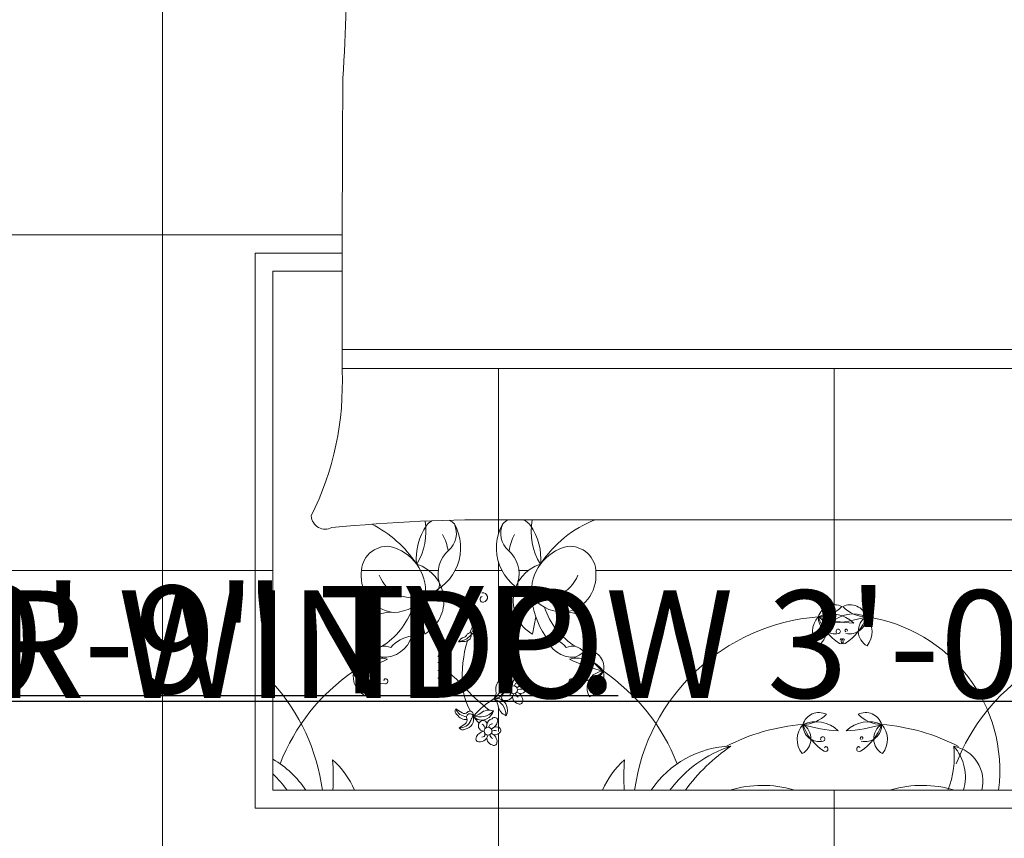
# Model space of a CAD drawing. Units: inches. Extents: x 351 to 1738, y -265 to 286.
# Tile 23 of 38: x 1127 to 1200, y 41 to 102. Entities that reach past the tile are written whole.
import ezdxf

# ---------------------------------------------------------------- set-up
doc = ezdxf.new("R2010")
doc.units = ezdxf.units.IN
doc.header["$MEASUREMENT"] = 0
for name, color, linetype, lineweight in [('A-ANNO-DIMS', 2, 'Continuous', 18), ('A-FLOR-PATT', 9, 'Continuous', 9), ('A-FURN', 18, 'Continuous', 13)]:
    doc.layers.add(name, color=color, linetype=linetype, lineweight=lineweight)
doc.styles.get("Standard").update_dxf_attribs({"font": 'arial.ttf'})
doc.dimstyles.get("Standard").update_dxf_attribs({"dimtxt": 8, "dimasz": 5, "dimexe": 0.18, "dimexo": 0.0625, "dimgap": 0.09, "dimtad": 1, "dimtoh": 1, "dimzin": 0, "dimdsep": 46, "dimlunit": 4, "dimtxsty": 'Standard', "dimcen": 0, "dimclre": 256, "dimadec": 0, "dimazin": 0, "dimtfac": 1, "dimtofl": 0, "dimtmove": 0, "dimatfit": 3, "dimfxl": 1, "dimtolj": 1, "dimtzin": 0, "dimlwe": -1, "dimarcsym": 0})

# ---------------------------------------------------------------- blocks, each defined once
blk = doc.blocks.new('*D52')
at = {"layer": 'A-ANNO-DIMS', "color": 0, "lineweight": -2, "transparency": 16777216}
for p, q in [((1098.304, 46.258), (1098.304, 51.258)), ((1098.304, 51.258), (1235.278, 51.258)), ((1098.304, 15.258), (1098.304, 41.258))]:
    blk.add_line(p, q, dxfattribs=at)
at = {"layer": 'A-ANNO-DIMS', "transparency": 16777216}
for p, q in [((1103.642, 46.258), (1098.124, 46.258)), ((1103.642, 10.258), (1098.124, 10.258))]:
    blk.add_line(p, q, dxfattribs=at)
at = {"layer": 'A-ANNO-DIMS', "color": 0, "transparency": 16777216}
for points in [[(1097.471, 41.258), (1099.137, 41.258), (1098.304, 46.258)], [(1097.471, 15.258), (1099.137, 15.258), (1098.304, 10.258)]]:
    blk.add_solid(points, dxfattribs=at)
at = {"layer": 'Defpoints', "color": 0, "transparency": 16777216}
for p in [(1098.304, 46.258), (1103.704, 46.258), (1103.704, 10.258)]:
    blk.add_point(p, dxfattribs=at)
at = {"layer": 'A-ANNO-DIMS', "color": 0, "transparency": 16777216, "insert": (1166.836, 55.49), "char_height": 8, "attachment_point": 5}
blk.add_mtext('\\A1;STAIR WINDOW 3\'-0" TYP.', dxfattribs=at)
blk = doc.blocks.new('*D53')
at = {"layer": 'A-ANNO-DIMS', "color": 0, "lineweight": -2, "transparency": 16777216}
for p, q in [((1098.704, 51.658), (1093.704, 51.658)), ((1117.704, 51.658), (1171.648, 51.658))]:
    blk.add_line(p, q, dxfattribs=at)
at = {"layer": 'A-ANNO-DIMS', "transparency": 16777216}
for p, q in [((1103.704, 46.321), (1103.704, 51.838)), ((1112.704, 46.321), (1112.704, 51.838))]:
    blk.add_line(p, q, dxfattribs=at)
at = {"layer": 'A-ANNO-DIMS', "color": 0, "transparency": 16777216}
for points in [[(1098.704, 52.492), (1098.704, 50.825), (1103.704, 51.658)], [(1117.704, 52.492), (1117.704, 50.825), (1112.704, 51.658)]]:
    blk.add_solid(points, dxfattribs=at)
at = {"layer": 'Defpoints', "color": 0, "transparency": 16777216}
for p in [(1112.704, 51.658), (1103.704, 46.258), (1112.704, 46.258)]:
    blk.add_point(p, dxfattribs=at)
at = {"layer": 'A-ANNO-DIMS', "color": 0, "transparency": 16777216, "insert": (1147.176, 55.833), "char_height": 8, "attachment_point": 5}
blk.add_mtext('\\A1;0\'-9" TYP.', dxfattribs=at)

msp = doc.modelspace()

# ---------------------------------------------------------------- hatches: boundary and pattern name
at = {"layer": 'A-FLOR-PATT', "transparency": 33554559}
h = msp.add_hatch(dxfattribs=at)
h.set_pattern_fill('ANSI37', color=256, scale=200, angle=135)
h.set_pattern_definition([(180, (1112.704, -164.037), (-2e-15, -25), []), (270, (1112.704, -164.037), (25, -5e-15), [])])
h.paths.add_polyline_path([(1380.064, 73.463), (1380.132, 148.463), (1338.064, 148.463), (1290.704, 148.463), (1290.704, 88.463), (1248.704, 88.463), (1248.704, -2.009), (1244.704, -2.009), (1244.704, 142.457), (1160.704, 142.457), (1160.704, 158.963), (1160.704, 170.137), (1160.704, 206.137), (1160.704, 228.963), (1112.704, 228.963), (1112.704, 209.963), (1112.704, 168.963), (1124.704, 168.963), (1124.704, 162.963), (1112.704, 162.963), (1112.704, 64.463), (1112.704, 60.463), (1112.704, 0.463), (1112.704, -48.026), (1146.804, -47.981), (1146.804, -35.691), (1207.804, -35.691), (1207.804, -47.902), (1236.542, -47.864), (1236.544, -50.009), (1248.5, -50.009), (1248.506, -102.915), (1248.512, -150.915), (1248.514, -164.037), (1248.549, -164.037), (1273.017, -164.037), (1273.017, -128.799), (1355.24, -128.799), (1355.24, -164.037), (1384.204, -164.037), (1384.204, -57.037), (1380.064, -57.037), (1380.064, -48.037), (1392.064, -48.037), (1392.064, -53.037), (1406.549, -53.037), (1406.549, -57.037), (1401.204, -57.037), (1401.204, -147.037), (1468.204, -147.037), (1468.204, -138.5), (1472.204, -138.5), (1472.204, -102.5), (1468.204, -102.5), (1468.204, -57.037), (1442.549, -57.037), (1442.549, -53.037), (1463.049, -53.037), (1463.049, -40.747), (1524.049, -40.747), (1524.049, -48.037), (1536.064, -48.037), (1536.064, -53.037), (1557.704, -53.037), (1557.704, 204.963), (1384.204, 204.963), (1384.204, 73.463), (1392.064, 73.463), (1392.064, 64.463), (1384.204, 64.463), (1384.204, -3.5), (1380.204, -3.537), (1380.204, 64.463), (1380.064, 64.463)])
h.paths.add_polyline_path([(1510.714, 86.458, -0.103984), (1511.661, 85.595, 0.470438), (1510.158, 87.614, 0.0961)], flags=16)
h.paths.add_polyline_path([(1510.443, 100.266, 0.009798), (1504.693, 100.48, 0.02879), (1504.6, 99.767, -0.165331), (1505.519, 96.135, -0.143601)], flags=16)
h.paths.add_polyline_path([(1487.201, 85.595, -0.103984), (1488.148, 86.458, 0.0961), (1488.704, 87.614, 0.470438)], flags=0)
h.paths.add_polyline_path([(1495.052, 100.43), (1494.178, 100.43, -0.026463), (1494.262, 99.774, -0.144219)], flags=16)
h.paths.add_polyline_path([(1444.485, 86.458, -0.103984), (1445.433, 85.595, 0.470438), (1443.93, 87.614, 0.0961)], flags=16)
h.paths.add_polyline_path([(1420.972, 85.595, -0.103984), (1421.92, 86.458, 0.0961), (1422.475, 87.614, 0.470438)], flags=16)
h.paths.add_polyline_path([(1428.632, 100.335, 0.001054), (1427.971, 100.309, -0.021524), (1428.033, 99.774, -0.114301)], flags=16)
h.paths.add_polyline_path([(1419.906, 143.708, 0.024979), (1420.222, 157.526), (1421.573, 159.101), (1421.573, 175.369), (1391.393, 175.369), (1391.393, 200.519), (1542.294, 200.519), (1542.294, 175.369), (1512.028, 175.369, 0.019865), (1511.521, 153.838, 0.025134), (1512.758, 118.323, 0.020553), (1512.942, 115.253), (1419.834, 115.253, -0.000414), (1419.843, 124.798), (1413.059, 124.798), (1413.059, 84.437, -0.061853), (1415.831, 80.45, -0.093077), (1420.972, 85.595, -0.267537), (1422.371, 84.732, 0.08511), (1424.052, 84.616, -0.885393), (1424.033, 84.851, -1.125815), (1424.073, 84.366, -0.087987), (1422.371, 84.732, -0.267537), (1422.326, 83.089, -0.370542), (1420.972, 85.595, 0.093077), (1415.831, 80.45, -0.087414), (1417.914, 73.937), (1418.941, 73.937, 0.02725), (1418.913, 76.906, -0.115703), (1421.051, 73.937), (1445.354, 73.937, -0.115703), (1447.492, 76.906, 0.02725), (1447.464, 73.937), (1448.491, 73.937, -0.087414), (1450.574, 80.45, 0.093077), (1445.433, 85.595, -0.370542), (1444.079, 83.089, -0.267537), (1444.034, 84.732, -0.087987), (1442.332, 84.366, -1.125815), (1442.372, 84.851, -2.032736), (1442.364, 84.368, 0.086378), (1444.034, 84.732, -0.267537), (1445.433, 85.595, -0.093077), (1450.574, 80.45, -0.257732), (1466.483, 90.927, -0.47867), (1468.832, 91.907, -0.47867), (1471.18, 90.927, -0.26264), (1483.053, 81.78, -0.071866), (1487.201, 85.595, -0.267537), (1488.6, 84.732, 0.08511), (1490.28, 84.616, -0.885393), (1490.262, 84.851, -1.125815), (1490.301, 84.366, -0.087987), (1488.6, 84.732, -0.267537), (1488.554, 83.089, -0.370542), (1487.201, 85.595, 0.071866), (1483.053, 81.78, -0.132065), (1484.143, 73.937), (1485.169, 73.937, 0.02725), (1485.142, 76.906, -0.115703), (1487.28, 73.937), (1511.582, 73.937, -0.115703), (1513.72, 76.906, 0.02725), (1513.693, 73.937), (1514.719, 73.937, -0.087414), (1516.802, 80.45, 0.093077), (1511.661, 85.595, -0.370542), (1510.308, 83.089, -0.267537), (1510.262, 84.732, -0.087987), (1508.561, 84.366, -1.125815), (1508.601, 84.851, -2.032736), (1508.592, 84.368, 0.086378), (1510.262, 84.732, -0.267537), (1511.661, 85.595, -0.093077), (1516.802, 80.45, -0.061853), (1519.575, 84.437), (1519.575, 73.937), (1413.059, 73.937), (1413.059, 124.798), (1419.843, 124.798, -0.000821)], flags=16)
h.paths.add_polyline_path([(1220.149, 54.133, -0.103984), (1220.869, 53.476, 0.470438), (1219.727, 55.011, 0.0961)], flags=16)
h.paths.add_polyline_path([(1219.944, 64.626, 0.009798), (1215.574, 64.789, 0.02879), (1215.503, 64.247, -0.165331), (1216.201, 61.487, -0.143601)], flags=16)
h.paths.add_polyline_path([(1209.779, 64.449, 0.097446), (1209.339, 64.751), (1208.247, 64.751, 0.12739), (1207.7, 64.326, 0.171586), (1206.95, 61.475, -0.158854), (1207.636, 59.45, 0.015898), (1207.795, 59.218, 0.061546), (1208.598, 59.616, 0.175416), (1208.638, 60.099, -0.284779), (1209.348, 62.472, 0.326216)], flags=16)
h.paths.add_polyline_path([(1169.818, 54.133, -0.103984), (1170.538, 53.476, 0.470438), (1169.396, 55.011, 0.0961)], flags=16)
h.paths.add_polyline_path([(1159.017, 62.472, 0.284764), (1158.307, 60.099, -0.175433), (1158.267, 59.616, 0.39293), (1159.448, 64.449, -0.32623)], flags=16)
h.paths.add_polyline_path([(1156.342, 58.239, -0.178321), (1154.011, 55.31, -0.174736), (1154.722, 55.233, -0.200802), (1156.27, 56.086, 0.12699), (1157.283, 58.991, -0.091205)], flags=16)
h.paths.add_polyline_path([(1156.624, 61.413, 0.157275), (1157.316, 64.247, 0.169622)], flags=16)
h.paths.add_polyline_path([(1152.67, 54.133, -0.0961), (1151.95, 53.476, 0.064076), (1154.465, 54.384, 0.199016)], flags=16)
h.paths.add_polyline_path([(1202.281, 53.476, -0.103984), (1203, 54.133, 0.0961), (1203.423, 55.011, 0.470438)], flags=0)
h.paths.add_polyline_path([(1151.139, 97.64, 0.024979), (1151.379, 108.141), (1152.406, 109.338), (1152.406, 121.701), (1129.47, 121.701), (1129.47, 140.814), (1244.149, 140.814), (1244.149, 121.701), (1221.148, 121.701, 0.019865), (1220.763, 105.338, 0.025134), (1221.703, 78.349, 0.020553), (1221.843, 76.016), (1151.078, 76.016, -0.128743), (1148.786, 65.037, 0.539352), (1150.327, 64.171, -0.027594), (1163.481, 64.751, 0.097695), (1163.04, 64.449, 0.326216), (1163.471, 62.472, -0.284777), (1164.181, 60.099, -0.194757), (1165.846, 61.443, -0.155402), (1165.172, 64.247, -0.166022), (1165.869, 61.475, -0.177014), (1167.852, 62.77, -0.448203), (1169.974, 60.807, -0.393499), (1167.679, 57.86, -0.895548), (1168.438, 54.524, -0.355767), (1166.218, 56.086, -0.066024), (1165.505, 57.539), (1165.251, 56.243, -0.371732), (1164.02, 59.758, -0.373614), (1163.04, 64.449, -0.097695), (1163.481, 64.751, 0.021354), (1153.294, 64.429, -0.134183), (1156.695, 61.368, 0.186873), (1154.636, 62.77, 0.448203), (1152.514, 60.807, 0.403726), (1154.905, 57.846, 0.711219), (1153.334, 55, 0.53154), (1151.95, 53.476, -0.267537), (1153.013, 52.821, 0.08511), (1154.29, 52.732, -0.885393), (1154.276, 52.911, -1.125815), (1154.306, 52.543, -0.087987), (1153.013, 52.821, -0.267537), (1152.978, 51.572, -0.370542), (1151.95, 53.476, 0.093077), (1148.043, 49.566, -0.087414), (1149.626, 44.617), (1150.406, 44.617, 0.02725), (1150.385, 46.873, -0.115703), (1152.01, 44.617), (1170.478, 44.617, -0.115703), (1172.103, 46.873, 0.02725), (1172.082, 44.617), (1172.862, 44.617, -0.087414), (1174.445, 49.566, 0.093077), (1170.538, 53.476, -0.370542), (1169.51, 51.572, -0.267537), (1169.475, 52.821, -0.087987), (1168.182, 52.543, -1.125815), (1168.212, 52.911, -2.032736), (1168.206, 52.544, 0.086378), (1169.475, 52.821, -0.267537), (1170.538, 53.476, -0.093077), (1174.445, 49.566, -0.257732), (1186.536, 57.528, -0.47867), (1188.321, 58.273, -0.47867), (1190.106, 57.528, -0.26264), (1199.128, 50.577, -0.071866), (1202.281, 53.476, -0.267537), (1203.344, 52.821, 0.08511), (1204.621, 52.732, -0.885393), (1204.607, 52.911, -1.125815), (1204.637, 52.543, -0.087987), (1203.344, 52.821, -0.267537), (1203.309, 51.572, -0.370542), (1202.281, 53.476, 0.071866), (1199.128, 50.577, -0.132065), (1199.957, 44.617), (1200.737, 44.617, 0.02725), (1200.716, 46.873, -0.115703), (1202.341, 44.617), (1220.809, 44.617, -0.115703), (1222.434, 46.873, 0.02725), (1222.413, 44.617), (1223.193, 44.617, -0.087414), (1224.776, 49.566, 0.093077), (1220.869, 53.476, -0.370542), (1219.841, 51.572, -0.267537), (1219.806, 52.821, -0.087987), (1218.513, 52.543, -1.125815), (1218.543, 52.911, -2.032736), (1218.537, 52.544, 0.086378), (1219.806, 52.821, -0.267537), (1220.869, 53.476, -0.093077), (1224.776, 49.566, -0.061853), (1226.883, 52.597), (1226.883, 44.617), (1145.936, 44.617), (1145.936, 83.269), (1151.091, 83.269, -0.000821)], flags=16)
h.paths.add_polyline_path([(1218.01, 57.86, -0.895548), (1218.769, 54.524, -0.355767), (1216.549, 56.086, -0.066024), (1215.836, 57.539), (1215.582, 56.243, -0.371732), (1214.351, 59.758, -0.373614), (1213.371, 64.449, 0.326216), (1213.802, 62.472, -0.284777), (1214.512, 60.099, -0.194757), (1216.177, 61.443, -0.179991), (1218.183, 62.77, -0.448203), (1220.305, 60.807, -0.393499)], flags=16)
h.paths.add_polyline_path([(1424.735, 91.363, -0.393499), (1421.715, 95.241, -0.448203), (1424.507, 97.824, -0.179991), (1427.147, 96.077, -0.194757), (1429.338, 94.309, -0.284777), (1430.272, 97.432, 0.326216), (1430.839, 100.034, -0.373614), (1429.55, 93.861, -0.371732), (1427.929, 89.235), (1427.596, 90.941, -0.066024), (1426.657, 89.029, -0.355767), (1423.736, 86.973, -0.895548)], flags=16)
h.paths.add_polyline_path([(1238.033, 131.257, -1), (1227.329, 131.257, -1)], flags=0)
h.paths.add_polyline_path([(1235.357, 131.257, -1), (1230.005, 131.257, -1)], flags=0)
h.paths.add_polyline_path([(1214.039, 54.243, 0.154382), (1214.38, 53.992, 0.358955), (1213.613, 54.016, 0.603948), (1214.379, 53.657, 0.371319), (1213.968, 52.872, 0.187994), (1214.312, 52.809, -0.592455), (1213.953, 52.967, -0.294279), (1214.083, 53.691, -1.300187), (1213.881, 54.134, -0.283762), (1214.469, 53.896, 1.15094)], flags=16)
h.paths.add_polyline_path([(1212.091, 56.286, -0.408434), (1211.337, 56.445, -0.036259), (1211.098, 56.848, -0.236098), (1211.59, 56.63, 0.035345), (1211.835, 56.543, -0.475241), (1212.091, 56.286, -0.475241), (1212.438, 56.182, 0.035345), (1212.631, 56.007, -0.236098), (1213.056, 55.676, -0.036259), (1212.588, 55.697, -0.408434)], flags=16)
h.paths.add_polyline_path([(1211.469, 50.297, 0.296043), (1210.47, 50.527, 0.310883), (1211.931, 50.148, 0.021255)], flags=16)
h.paths.add_polyline_path([(1213.739, 51.818, -0.036259), (1213.271, 51.838, -0.408434), (1212.774, 52.427, -0.094786), (1212.293, 50.703, 1.150474), (1212.911, 50.232, 0.166288), (1213.265, 50.68, -0.025254), (1212.603, 50.13, 1.087932), (1212.471, 49.407, 0.166288), (1213.02, 49.251, -0.016128), (1212.567, 49.563, -0.286859), (1212.217, 49.638, 0.022156), (1212.046, 50.055, -0.64613), (1212.185, 50.498, 0.088412), (1212.732, 52.077, -1.186037), (1213.121, 52.323, 0.035345), (1213.314, 52.148, -0.236098)], flags=16)
h.paths.add_polyline_path([(1212.094, 50.342, -0.048524), (1211.54, 49.605, -1.103834), (1211.397, 48.738, -0.785515), (1211.683, 48.254, -0.392043), (1210.948, 48.525, -0.392819), (1210.561, 47.995, -0.592455), (1210.201, 48.153, -0.294279), (1210.331, 48.877, -0.704172), (1210.316, 49.592, -0.679344), (1210.729, 50.112, 0.563676)], flags=16)
h.paths.add_polyline_path([(1211.274, 49.829, -0.139826), (1210.745, 49.859, -0.217879), (1210.948, 49.509, -0.498572)], flags=0)
h.paths.add_polyline_path([(1433.426, 81.49, -0.181571), (1434.245, 81.788, -0.008067), (1433.726, 82.205, 0.045578), (1432.755, 81.242, 0.179011)], flags=16)
h.paths.add_polyline_path([(1434.146, 81.009, -0.132442), (1433.645, 80.771, 0.259089), (1433.234, 80.471, -0.180211), (1433.392, 80.805, -0.16994), (1432.758, 81.109, 0.032652), (1433.273, 80.474, -0.493363), (1434.046, 80.146, -0.390497)], flags=16)
h.paths.add_polyline_path([(1434.83, 80.047, -0.947538), (1435.294, 79.576, -0.299128), (1434.625, 79.404, -0.270439), (1435.01, 78.591, -0.592455), (1434.537, 78.382, -0.392819), (1434.027, 79.08, -0.392043), (1433.06, 78.723, -0.352042), (1433.003, 79.197, -0.197216), (1433.75, 79.734, -0.71364), (1434.447, 79.939, -0.21479), (1434.819, 80.475, 0.408833), (1435.075, 80.803, -0.226152)], flags=16)
h.paths.add_polyline_path([(1432.67, 81.217, -0.454218), (1431.897, 79.923, -0.414411), (1431.301, 80.035, 0.016129), (1431.897, 80.445, 0.27957), (1432.073, 80.871, -0.289504), (1431.103, 81.321, -0.414411), (1430.978, 81.915, 0.01613), (1431.586, 81.521, 0.341293), (1432.125, 81.583, -0.813186)], flags=16)
h.paths.add_polyline_path([(1429.893, 86.381, -0.947538), (1430.358, 85.91, -0.173106), (1429.984, 85.712, -0.038817), (1431.625, 84.214, -0.0879), (1432.097, 88.549, -0.049768), (1431.254, 88.49, -0.236098), (1431.814, 88.925, 0.035345), (1432.067, 89.155, -0.475241), (1432.524, 89.291, -0.475241), (1432.86, 89.63, 0.035345), (1433.182, 89.744, -0.236098), (1433.83, 90.032, -0.036259), (1433.516, 89.502, -0.408434), (1432.524, 89.291, -0.312424), (1432.106, 88.58, 0.088559), (1431.625, 84.214, -0.408434), (1430.971, 83.439, -0.036259), (1430.355, 83.412, -0.236098), (1430.914, 83.847, 0.035345), (1431.168, 84.078, -0.475241), (1431.625, 84.214, 0.038817), (1429.984, 85.712, -0.321732), (1429.333, 86.048, -0.32743), (1429.883, 86.809, 0.408833), (1430.138, 87.138, -0.226152)], flags=16)
h.paths.add_polyline_path([(1211.206, 58.616, -0.999784), (1211.336, 59.323, -0.614994)], flags=16)
h.paths.add_polyline_path([(1210.288, 49.429, 0.154382), (1210.629, 49.178, 0.358955), (1209.861, 49.202, 0.603948), (1210.627, 48.843, -0.534825), (1210.806, 49.295, 0.748346)], flags=16)
h.paths.add_polyline_path([(1209.589, 51.828, -0.008791), (1209.775, 51.753, 0.112231), (1209.466, 52.019, 1.418851), (1209.014, 51.708, -0.458726), (1208.651, 51.073, -0.592455), (1208.291, 51.232, -0.294279), (1208.421, 51.955, -1.300187), (1208.219, 52.398, -0.226005), (1208.719, 52.257, -0.475519), (1209.158, 52.369, -1.455499), (1209.603, 52.664, 0.421305), (1209.191, 52.262, -0.591212), (1208.979, 51.796, 0.497399), (1209.773, 51.333, 0.649312)], flags=16)
h.paths.add_polyline_path([(1208.029, 52.041, 0.544667), (1208.832, 52.045, 0.220132)], flags=0)
h.paths.add_polyline_path([(1210.438, 51.425, -0.2042), (1210.277, 52.018, 0.270826), (1209.915, 52.897, 0.324115)], flags=0)
h.paths.add_polyline_path([(1209.668, 52.407, -0.60139), (1208.99, 52.221, -0.394916), (1208.248, 52.83, -0.836792), (1208.651, 53.017, -0.338488), (1209.039, 52.571, 0.194138), (1209.191, 52.262, 0.413995), (1209.712, 52.475, 0.51771), (1210.503, 51.416, 0.401922), (1209.493, 50.93, 0.206396), (1209.516, 50.165, -0.319463), (1210.417, 51.418, -0.466635)], flags=16)
h.paths.add_polyline_path([(1206.601, 56.086, -0.355767), (1204.381, 54.524, -0.921198), (1205.236, 57.846, 0.206569), (1207.614, 58.991, -0.12699)], flags=16)
h.paths.add_polyline_path([(1435.487, 82.816, 0.527765), (1436.615, 83.361, 0.50854), (1437.05, 82.433, 0.592455), (1437.524, 82.641, 0.331245), (1436.963, 83.548, 0.387863), (1437.808, 83.626, 0.592954), (1437.618, 84.176, 0.226016), (1436.961, 83.99, 0.318205), (1437.588, 84.854, 0.689374), (1437.05, 84.991, 0.335765), (1436.539, 84.41, -0.156993), (1436.404, 84.065, -0.434611), (1436.961, 83.99, -0.21479), (1437.333, 84.526, 0.408833), (1437.588, 84.854, -0.226152), (1437.343, 84.097, -0.947538), (1437.808, 83.626, -0.299128), (1437.139, 83.455, -0.270439), (1437.524, 82.641, -0.592455), (1437.05, 82.433, -0.392819), (1436.541, 83.13, -0.43966), (1435.475, 82.794, -0.174614), (1435.942, 82.244, -0.206396), (1435.912, 81.237, -0.270826), (1435.125, 82.208, 0.207976), (1434.686, 82.904, -0.196495)], flags=16)
h.paths.add_polyline_path([(1435.386, 84.832, 0.270811), (1434.91, 83.676, -0.204217), (1434.699, 82.895, 0.324115)], flags=0)
h.paths.add_polyline_path([(1435.68, 84.18, -0.217656), (1435.554, 83.304, -0.176705), (1436.236, 83.778, -0.373036)], flags=0)
h.paths.add_polyline_path([(1435.566, 100.034, 0.326216), (1436.133, 97.432, -0.284777), (1437.067, 94.309, -0.194757), (1439.258, 96.077, -0.155402), (1438.371, 99.767, -0.166022), (1439.289, 96.12, -0.177014), (1441.897, 97.824, -0.448203), (1444.69, 95.241, -0.393499), (1441.67, 91.363, -0.895548), (1442.669, 86.973, -0.355767), (1439.748, 89.029, -0.066024), (1438.809, 90.941), (1438.476, 89.235, -0.371732), (1436.855, 93.861, -0.373614)], flags=16)
h.paths.add_polyline_path([(1191.252, 49.507, -0.274022), (1190.658, 48.409, 0.267537), (1191.311, 47.344, 0.370542)], flags=0)
h.paths.add_polyline_path([(1190.301, 49.717, 0.199016), (1188.619, 49.04, 0.064076), (1191.252, 49.507, -0.0961)], flags=0)
h.paths.add_polyline_path([(1189.518, 47.857, 1.125815), (1189.676, 47.523, 2.044605)], flags=0)
h.paths.add_polyline_path([(1464.974, 80.372, 0.274022), (1465.756, 78.927, -0.083013)], flags=0)
h.paths.add_polyline_path([(1464.974, 80.372, 0.370542), (1464.897, 77.525, 0.576324)], flags=0)
h.paths.add_polyline_path([(1464.974, 80.372, -0.470438), (1467.284, 81.372, -0.0961), (1466.226, 80.648, -0.199016), (1468.439, 79.757, -0.064076)], flags=0)
h.paths.add_polyline_path([(1189.511, 56.43, -0.259467), (1188.321, 56.391, -0.259467), (1187.13, 56.43, 0.08511), (1188.193, 55.716, -0.885393), (1188.27, 55.878, -1.196013), (1188.355, 55.442, 0.101459)], flags=0)
h.paths.add_polyline_path([(1188.321, 57.596, 0.078072), (1187.678, 57.24, 0.01555), (1188.321, 57.136, 0.01555), (1188.964, 57.24, 0.078072)], flags=0)
h.paths.add_polyline_path([(1190.164, 55.365, -0.576324), (1190.106, 57.528, -0.198294), (1188.321, 58.319, -0.198294), (1186.536, 57.528, -0.576324), (1186.477, 55.365, -0.370542), (1186.536, 57.528, 0.198294), (1188.321, 58.319, 0.198294), (1190.106, 57.528, -0.370542)], flags=0)
h.paths.add_polyline_path([(1188.372, 55.878, 1.125814), (1188.529, 55.544, 2.044605)], flags=0)
h.paths.add_polyline_path([(1186.341, 49.717, -0.0961), (1185.389, 49.507, 0.064076), (1188.022, 49.04, 0.199016)], flags=0)
h.paths.add_polyline_path([(1185.389, 49.507, -0.267537), (1185.984, 48.409, 0.08511), (1187.046, 47.695, -0.885393), (1187.123, 47.857, -1.125815), (1186.966, 47.523, -0.087987), (1185.984, 48.409, -0.267537), (1185.331, 47.344, -0.370542)], flags=0)
h.paths.add_polyline_path([(1399.441, 187.944, -1), (1413.525, 187.944, -1)], flags=0)
h.paths.add_polyline_path([(1402.962, 187.944, -1), (1410.004, 187.944, -1)], flags=0)
h.paths.add_polyline_path([(1357.663, -72.245), (1377.272, -72.245), (1377.272, -91.854), (1357.663, -91.854)], flags=16)
h.paths.add_polyline_path([(1467.256, 78.201, -1.125815), (1467.049, 77.761, -2.044605)], flags=0)
h.paths.add_polyline_path([(1468.822, 88.714, 0.941125), (1469.106, 88.316, 1.137152), (1468.765, 88.755, 0.890986), (1468.99, 88.245, 0.094828), (1470.398, 89.481, -0.267537), (1471.18, 90.927, -0.028123), (1469.678, 90.547, -0.028774), (1469.948, 90.311, -0.020327), (1468.832, 90.41, -0.020327), (1467.716, 90.311, -0.028774), (1467.986, 90.547, -0.028123), (1466.483, 90.927, -0.267537), (1467.265, 89.481, 0.08511), (1468.663, 88.542, -1.202316)], flags=0)
h.paths.add_polyline_path([(1178.25, 124.523, -0.119929), (1165.65, 124.145, -0.107349), (1159.133, 124.446, -0.102891), (1159.132, 130.465, -0.074897), (1158.993, 137.956, 0.002027), (1167.844, 137.479, -0.07553), (1180.337, 137.666, -0.075861), (1186.502, 137.688, -0.14099), (1186.272, 130.046, -0.095481), (1186.729, 124.748, -0.10603)], flags=0)
h.paths.add_polyline_path([(1469.225, 79.757, -0.199016), (1471.437, 80.648, -0.0961), (1470.379, 81.372, -0.470438), (1472.689, 80.372, -0.370542), (1472.766, 77.525, -0.267537), (1471.907, 78.927, -0.087986), (1470.615, 77.761, -1.125849), (1470.408, 78.201, -2.032736), (1470.642, 77.778, 0.086378), (1471.907, 78.927, -0.267537), (1472.689, 80.372, -0.064076)], flags=0)
h.paths.add_polyline_path([(1430.423, 186.902, -0.074897), (1430.24, 196.758, 0.002027), (1441.887, 196.131, -0.07553), (1458.326, 196.377, -0.075861), (1466.438, 196.406, -0.14099), (1466.136, 186.35, -0.095481), (1466.737, 179.378, -0.10603), (1455.58, 179.082, -0.119929), (1439, 178.585, -0.107349), (1430.425, 178.981, -0.102891)], flags=0)
h.paths.add_polyline_path([(1162.258, 49.939, 0.335765), (1161.87, 49.497, -0.156994), (1161.767, 49.235, -0.434611), (1162.19, 49.178, -0.21479), (1162.473, 49.585, 1.529195)], flags=16)
h.paths.add_polyline_path([(1161.683, 49.021, 0.581518), (1161.268, 49.583, 0.592761)], flags=16)
h.paths.add_polyline_path([(1162.602, 48.058, 0.371319), (1162.192, 48.843, 0.434533), (1162.88, 48.962, 0.185081), (1162.197, 48.926, 1.121837)], flags=16)
h.paths.add_polyline_path([(1161.443, 48.941, -1.307104), (1161.495, 48.571, -0.217752), (1161.136, 48.254, 0.697303), (1161.871, 49.048, 0.121514)], flags=16)
h.paths.add_polyline_path([(1162.531, 49.429, -0.207084), (1162.05, 49.146, -0.99203)], flags=16)
h.paths.add_polyline_path([(1161.304, 49.578, -0.719667), (1161.513, 50.079, -0.130428), (1160.836, 50.168, 0.039593)], flags=0)
h.paths.add_polyline_path([(1162.036, 50.584, -0.008067), (1161.642, 50.9, 0.029367), (1161.35, 50.297, -0.205788)], flags=16)
h.paths.add_polyline_path([(1162.882, 51.392, -0.124733), (1162.763, 51.828, -0.101191), (1162.399, 51.438, -0.153425)], flags=0)
h.paths.add_polyline_path([(1164.235, 51.85, -0.309107), (1164.513, 51.136, -0.627125), (1163.781, 51.603, -0.685909), (1162.777, 51.219, -0.233285), (1163.303, 50.165, -0.270826), (1162.705, 50.903, 0.2042), (1162.381, 51.425, 0.204182), (1162.542, 52.018, -0.270841), (1162.903, 52.897, -0.127261), (1163.219, 52.529, -1.168681), (1163.781, 52.587, -0.329112), (1164.168, 53.017, -0.836792), (1164.571, 52.83, -0.193341), (1164.391, 52.338, -0.947538), (1164.744, 51.981, -0.299128)], flags=16)
h.paths.add_polyline_path([(1163.598, 51.937, -1.262956), (1163.236, 51.831, 0.012575), (1162.971, 51.721, 0.230657), (1163.151, 52.407, -0.164898), (1163.178, 52.661, -0.44932), (1163.628, 52.262, -0.721477), (1164.154, 52.088, -0.849998)], flags=0)
h.paths.add_polyline_path([(1161.613, 58.616, -0.980413), (1161.525, 59.049, -2.908935)], flags=16)
h.paths.add_polyline_path([(1160.252, 49.166, -0.414411), (1159.799, 49.251, 0.016129), (1160.252, 49.563, 0.27957), (1160.386, 49.887, -0.289504), (1159.649, 50.229, -0.414411), (1159.554, 50.68, 0.01613), (1160.015, 50.381, 0.617885), (1160.526, 50.703, -0.094786), (1160.045, 52.427, -0.140444), (1159.682, 52.042, -0.057856), (1159.3, 51.872, 0.544843), (1160.046, 52.419, -0.088122), (1160.404, 55.721, -0.049768), (1159.763, 55.676, -0.236098), (1160.188, 56.007, 0.035345), (1160.381, 56.182, -0.475241), (1160.728, 56.286, -0.475241), (1160.984, 56.543, 0.035345), (1161.229, 56.63, -0.236098), (1161.721, 56.848, -0.036259), (1161.482, 56.445, -0.408434), (1160.728, 56.286, -0.312424), (1160.411, 55.745, 0.088559), (1160.045, 52.427, 0.107081), (1160.634, 50.498, -0.494798), (1160.839, 50.149, -0.454218)], flags=16)
h.paths.add_polyline_path([(1160.666, 49.808, -2.076528), (1160.828, 50.172, 0.019586)], flags=0)
h.paths.add_polyline_path([(1158.439, 53.992, 0.154382), (1158.78, 54.243, 0.748346), (1158.262, 54.109, -0.338225), (1158.492, 53.839, -0.170816), (1159.124, 53.779, 0.495729), (1158.938, 54.134, 0.226016)], flags=16)
h.paths.add_polyline_path([(1160.045, 52.427, 0.038817), (1158.798, 53.565, -0.119818), (1158.574, 53.586, -0.309107), (1158.851, 52.872, -0.187994), (1158.506, 52.809, 0.592455), (1158.866, 52.967, 0.331245), (1158.44, 53.657, 0.201245), (1158.798, 53.565, -0.034023), (1159.901, 52.578, -0.044253), (1159.698, 52.323, -0.475241)], flags=16)
h.paths.add_polyline_path([(1336.926, -95.392), (1336.926, -117.945), (1291.82, -117.945), (1291.82, -95.392)], flags=16)
h.paths.add_polyline_path([(1357.535, -97.244), (1357.726, -96.697, 0.034844)], flags=16)
h.paths.add_polyline_path([(1376.693, -96.478), (1377.301, -96.5, 0.031497), (1375.907, -96.424), (1357.726, -96.424)], flags=16)
h.paths.add_polyline_path([(1379.403, -119.667, 0.026706), (1380.043, -119.439, -0.015299)], flags=16)
h.paths.add_polyline_path([(1357.726, -120.202), (1357.821, -120.202), (1357.821, -120.201)], flags=16)
h.paths.add_polyline_path([(1354.171, -104.592), (1354.469, -98.672, 0.011138)], flags=16)
h.paths.add_polyline_path([(1355.058, -119.136), (1354.578, -118.539, 0.143164)], flags=16)
h.paths.add_polyline_path([(1378.851, -96.821), (1378.85, -96.82), (1378.85, -96.82, -0.04968), (1380.055, -97.191), (1378.85, -96.82, 0.150054), (1375.135, -97.188), (1375.136, -119.44, -0.00997), (1374.747, -116.649), (1357.726, -116.649, 0.169385), (1357.535, -119.382), (1357.535, -119.382), (1357.535, -119.382, 0.034818), (1357.726, -119.928), (1357.726, -119.928), (1357.726, -119.929, -0.034877), (1357.535, -119.382), (1355.507, -119.382), (1355.317, -119.278), (1357.535, -119.382, -0.169394), (1357.726, -116.649, -0.039151), (1374.686, -116.113, -0.002015), (1374.625, -115.546, 0.115322), (1369.915, -115.474, 0.060921), (1369.922, -101.154, 0.115146), (1374.625, -101.079, -0.002016), (1374.686, -100.513, -0.039151), (1357.726, -99.977), (1374.747, -99.977, -0.009963), (1375.135, -97.188), (1375.135, -97.188, -0.150108)], flags=16)
h.paths.add_polyline_path([(1490.963, 91.363, -0.393499), (1487.944, 95.241, -0.448203), (1490.736, 97.824, -0.179991), (1493.376, 96.077, -0.194757), (1495.567, 94.309, -0.284777), (1496.501, 97.432, 0.326216), (1497.068, 100.034, -0.373614), (1495.778, 93.861, -0.371732), (1494.158, 89.235), (1493.824, 90.941, -0.066024), (1492.886, 89.029, -0.355767), (1489.964, 86.973, -0.895548)], flags=16)
h.paths.add_polyline_path([(1354.86, -97.658), (1355.316, -97.348, 0.101911)], flags=16)
h.paths.add_polyline_path([(1497.063, 83.327, 0.176724), (1496.37, 83.785, -0.405139), (1496.016, 83.384, 0.497399), (1497.06, 82.774, 0.649312), (1496.818, 83.426, -0.008791)], flags=16)
h.paths.add_polyline_path([(1496.339, 83.783, 0.592761), (1496.886, 84.522, 0.581518)], flags=16)
h.paths.add_polyline_path([(1495.11, 82.641, 0.592455), (1495.583, 82.433, 0.676915), (1495.805, 83.59, 0.375669)], flags=16)
h.paths.add_polyline_path([(1495.015, 84.176, -0.145057), (1495.301, 84.526, -0.408833), (1495.045, 84.854, 0.220629), (1495.381, 84.152, -0.199594), (1495.851, 83.764, -0.524017), (1494.826, 83.626, -0.592998)], flags=16)
h.paths.add_polyline_path([(1501.655, 81.915, -0.016129), (1501.048, 81.521, -0.392719), (1500.462, 81.37, -0.21067), (1500.607, 81.142, 0.306699)], flags=16)
h.paths.add_polyline_path([(1500.11, 89.291, -0.408434), (1499.118, 89.502, -0.036259), (1498.803, 90.032, -0.236098), (1499.451, 89.744, 0.035345), (1499.774, 89.63, -0.475241), (1500.11, 89.291, -0.475241), (1500.567, 89.155, 0.035345), (1500.82, 88.925, -0.236098), (1501.379, 88.49, -0.036259), (1500.763, 88.516, -0.408434)], flags=16)
h.paths.add_polyline_path([(1498.908, 82.205, -0.051322), (1500.013, 81.134, -0.587931), (1500.234, 81.676, 0.107081), (1501.009, 84.214, -0.03529)], flags=16)
h.paths.add_polyline_path([(1496.93, 83.875, -0.206396), (1497.247, 84.832, -0.270826), (1497.724, 83.676, 0.207976), (1497.944, 82.884, -0.381455)], flags=16)
h.paths.add_polyline_path([(1496.721, 81.237, 0.270812), (1497.509, 82.208, -0.204216), (1497.935, 82.895, 0.324115)], flags=16)
h.paths.add_polyline_path([(1497.529, 80.125, -0.145057), (1497.814, 80.475, -0.703182), (1498.282, 81.178, -0.122925), (1497.977, 81.714, -0.270837), (1499.207, 81.49, 0.207964), (1499.993, 81.248, -0.265145), (1499.278, 80.472, 0.381901), (1498.808, 79.947, -0.305905), (1498.848, 79.519, 0.499482), (1498.574, 79.217, -0.458726), (1498.097, 78.382, -0.592455), (1497.624, 78.591, -0.270439), (1498.009, 79.404, -0.299116), (1497.34, 79.576, -0.593016)], flags=16)
h.paths.add_polyline_path([(1500.736, 79.923, 0.414411), (1501.333, 80.035, -0.321648), (1500.192, 80.765, 0.019886), (1499.976, 81.251, 0.465331)], flags=16)
h.paths.add_polyline_path([(1501.009, 84.214, -0.038817), (1502.649, 85.712, -0.173095), (1502.276, 85.91, -0.593016), (1502.465, 86.46, -0.145057), (1502.751, 86.809, -0.408833), (1502.495, 87.138, 0.220629), (1502.831, 86.436, -0.199594), (1503.301, 86.048, -0.321732), (1502.649, 85.712, 0.038817), (1501.009, 84.214, 0.122449), (1501.412, 83.755, 0.475491), (1501.335, 84.226, 0.055822), (1501.719, 83.847, -0.236098), (1502.278, 83.412, -0.036259), (1501.663, 83.439, -0.408434)], flags=16)
h.paths.add_polyline_path([(1501.794, 100.034, 0.326216), (1502.362, 97.432, -0.284777), (1503.295, 94.309, -0.194757), (1505.486, 96.077, -0.179991), (1508.126, 97.824, -0.448203), (1510.918, 95.241, -0.393499), (1507.899, 91.363, -0.895548), (1508.898, 86.973, -0.355767), (1505.976, 89.029, -0.066024), (1505.038, 90.941), (1504.704, 89.235, -0.371732), (1503.084, 93.861, -0.373614)], flags=16)
h.paths.add_polyline_path([(1146.29, 131.257, -1), (1135.587, 131.257, -1)], flags=0)
h.paths.add_polyline_path([(1143.614, 131.257, -1), (1138.262, 131.257, -1)], flags=0)
h.paths.add_polyline_path([(1524.064, 73.463), (1536.064, 73.463), (1536.064, 64.463), (1524.064, 64.463)], flags=16)
h.paths.add_polyline_path([(1520.162, 187.944, -1), (1534.246, 187.944, -1)], flags=0)
h.paths.add_polyline_path([(1530.725, 187.944), (1527.204, 187.944), (1527.204, 184.423, 0.414214)], flags=0)
h.paths.add_polyline_path([(1278.415, -91.154), (1331.067, -91.154), (1331.067, -80.583), (1278.415, -80.583)], flags=24)
h.paths.add_polyline_path([(1266.655, -79.354), (1354.738, -79.354), (1354.738, -67.817), (1266.655, -67.817)], flags=24)
h.paths.add_polyline_path([(1115.482, 206.184), (1155.098, 206.184), (1155.098, 217.714), (1115.482, 217.714)], flags=24)
h.paths.add_polyline_path([(1161.771, 8.501), (1222.466, 8.501), (1222.466, 19.079), (1161.771, 19.079)], flags=24)
h.paths.add_polyline_path([(1164.656, 18.795), (1210.615, 18.795), (1210.615, 30.324), (1164.656, 30.324)], flags=24)
h.paths.add_polyline_path([(1368.147, -32.882), (1379.362, -32.882), (1379.362, -21.733), (1368.147, -21.733)], flags=24)
h.paths.add_polyline_path([(1244.842, -31.012), (1256.057, -31.012), (1256.057, -19.863), (1244.842, -19.863)], flags=24)
h.paths.add_polyline_path([(1114.589, 195.739), (1156.517, 195.739), (1156.517, 206.31), (1114.589, 206.31)], flags=24)
h.paths.add_polyline_path([(1436.398, 37.632), (1505.131, 37.632), (1505.131, 48.203), (1436.398, 48.203)], flags=24)
h.paths.add_polyline_path([(1435.991, 47.919), (1507.906, 47.919), (1507.906, 59.456), (1435.991, 59.456)], flags=24)
h.paths.add_polyline_path([(1415.107, -124.896), (1457.038, -124.896), (1457.038, -114.318), (1415.107, -114.318)], flags=24)
h.paths.add_polyline_path([(1417.992, -114.602), (1457.609, -114.602), (1457.609, -103.073), (1417.992, -103.073)], flags=24)

# ---------------------------------------------------------------- linework, layer by layer
at = {"layer": 'A-FURN'}
for p, q in [((1221.734, 77.446), (1151.085, 77.446)), ((1221.843, 76.016), (1151.085, 76.016)), ((1210.09, 64.751), (1163.529, 64.751)), ((1157.237, 56.243), (1156.983, 57.539)), ((1165.251, 56.243), (1165.505, 57.539))]:
    msp.add_line(p, q, dxfattribs=at)
msp.add_lwpolyline([(1151.139, 97.64, 0.001242), (1151.085, 75.881, -0.127202), (1148.786, 65.037)], format="xyb", dxfattribs=at)
for points in [[(1221.852, 84.598), (1228.212, 84.598), (1228.212, 43.288), (1144.607, 43.288), (1144.607, 84.598), (1151.094, 84.598)], [(1151.091, 83.269), (1145.936, 83.269), (1145.936, 44.617), (1226.883, 44.617), (1226.883, 83.269), (1221.828, 83.269)]]:
    msp.add_lwpolyline(points, dxfattribs=at)
for centre in [(1163.862, 52.088), (1161.952, 49.009)]:
    msp.add_circle(centre, 0.292, dxfattribs=at)
for centre, radius, start, end in [((1046.231, 105.29), 105.187, 355.82941, 1.55305), ((1149.841, 65.111), 1.058, 183.97998, 297.34124), ((1162.161, -54.623), 119.381, 89.34325, 95.68869), ((1152.577, 63.902), 4.751, 328.82178, 9.15542), ((1158.462, 63.482), 1.381, 120.0293, 142.32497), ((1158.462, 63.482), 1.381, 44.45169, 63.55801), ((1164.026, 63.482), 1.381, 113.22901, 135.54831), ((1164.026, 63.482), 1.381, 37.67503, 66.71436), ((1169.911, 63.902), 4.751, 169.71335, 211.17822), ((1173.094, 56.675), 8.679, 111.49413, 146.33288), ((1149.394, 56.675), 8.679, 33.66712, 63.29966), ((1161.026, 61.839), 4.423, 145.78505, 184.73037), ((1156.257, 62.668), 3.655, 289.28218, 29.1751), ((1157.878, 63.756), 1.716, 311.56531, 23.83541), ((1166.231, 62.668), 3.655, 150.8249, 250.71782), ((1164.61, 63.756), 1.716, 156.16459, 228.43469), ((1161.462, 61.839), 4.423, 355.26963, 34.21495), ((1155.705, 62.007), 3.296, 7.43599, 29.91487), ((1166.783, 62.007), 3.296, 150.08513, 172.56401), ((1154.45, 60.843), 1.936, 84.48557, 181.05378), ((1153.856, 59.41), 3.449, 355.29334, 76.921), ((1160.577, 60.713), 2.351, 131.56531, 195.14713), ((1161.911, 60.713), 2.351, 344.85287, 48.43469), ((1168.632, 59.41), 3.449, 103.079, 184.70666), ((1168.038, 60.843), 1.936, 358.94622, 95.51443), ((1155.815, 58.714), 2.851, 299.90854, 73.1337), ((1166.673, 58.714), 2.851, 106.8663, 240.09146), ((1155.244, 60.566), 2.74, 174.94485, 262.88575), ((1156.321, 61.605), 2.661, 201.58187, 291.42215), ((1166.167, 61.605), 2.661, 248.57785, 338.41813), ((1167.244, 60.566), 2.74, 277.11425, 5.05515), ((1161.026, 61.839), 4.423, 212.70113, 216.34448), ((1157.62, 59.913), 0.712, 257.30406, 15.14713), ((1164.868, 59.913), 0.712, 164.85287, 282.69594), ((1161.462, 61.839), 4.423, 323.65552, 327.29887), ((1154.768, 61.175), 3.331, 272.3591, 324.04014), ((1151.151, 59.502), 6.154, 326.28828, 356.5076), ((1161.573, 58.833), 0.221, 102.70507, 280.43845), ((1161.548, 58.969), 0.359, 280.43845, 100.41356), ((1167.72, 61.175), 3.331, 215.95986, 267.6409), ((1171.337, 59.502), 6.154, 183.4924, 213.71172), ((1151.201, 59.938), 5.414, 301.26137, 341.7045), ((1171.287, 59.938), 5.414, 198.2955, 238.73863), ((1187.728, 57.182), 1.241, 63.02737, 163.80375), ((1186.471, 60.085), 2.558, 271.45846, 315.37266), ((1188.913, 57.182), 1.241, 16.19625, 116.97263), ((1190.171, 60.085), 2.558, 224.62734, 268.54154), ((1154.614, 56.15), 1.721, 80.26398, 250.86884), ((1169.522, 53.061), 9.498, 153.0032, 159.89408), ((1167.874, 56.15), 1.721, 289.13116, 99.73602), ((1187.701, 42.599), 14.975, 94.46233, 172.25504), ((1187.766, 56.413), 1.661, 137.78732, 219.11446), ((1185.88, 56.464), 1.251, 298.5391, 58.36268), ((1187.76, 57.481), 1.225, 177.75849, 283.85198), ((1187.511, 55.371), 2.368, 45.54113, 114.31008), ((1189.67, 67.525), 10.476, 252.59304, 267.25817), ((1190.119, 58.756), 3.787, 198.91595, 238.01098), ((1189.131, 55.371), 2.368, 65.68992, 134.45887), ((1186.972, 67.525), 10.476, 272.74183, 287.40696), ((1186.523, 58.756), 3.787, 301.98902, 341.08405), ((1188.881, 57.481), 1.225, 256.14802, 2.24151), ((1190.762, 56.464), 1.251, 121.63732, 241.4609), ((1188.876, 56.413), 1.661, 320.88554, 42.21268), ((1188.456, 46.057), 11.59, 352.86355, 81.81966), ((1160.961, 56.31), 0.234, 84.37838, 186.05427), ((1160.491, 58.318), 1.842, 285.51291, 293.60991), ((1161.693, 56.247), 0.602, 87.35788, 140.49441), ((1160.301, 57.975), 1.813, 301.16403, 321.56124), ((1158.827, 58.292), 3.234, 324.68979, 333.49364), ((1188.015, 56.448), 0.162, 283.85198, 219.92454), ((1188.612, 56.511), 0.0976, 320.19092, 256.02088), ((1154.201, 56.668), 2.149, 265.96902, 344.3045), ((1156.516, 53.811), 2.289, 96.1662, 141.58255), ((1160.307, 55.417), 0.602, 101.32561, 154.46214), ((1159.441, 57.46), 1.813, 280.25878, 300.65599), ((1169.522, 53.061), 9.498, 163.58418, 183.82768), ((1159.049, 57.455), 1.842, 308.21012, 316.30712), ((1160.179, 56.244), 0.55, 278.34322, 4.28685), ((1159.875, 56.727), 0.961, 300.65599, 332.63414), ((1160.597, 56.092), 0.234, 55.76575, 157.44165), ((1160.742, 57.247), 0.961, 269.18588, 301.16403), ((1161.024, 56.75), 0.55, 237.53317, 323.47681), ((1165.972, 53.811), 2.289, 38.41745, 83.8338), ((1168.287, 56.668), 2.149, 195.6955, 274.03098), ((1188.211, 55.702), 0.186, 238.01098, 71.55918), ((1188.241, 55.793), 0.0903, 71.55918, 188.01668), ((1188.431, 55.702), 0.186, 108.44082, 301.98902), ((1188.4, 55.793), 0.0903, 351.98332, 108.44082), ((1153.156, 53.771), 1.241, 92.95159, 193.72796), ((1150.618, 55.66), 2.558, 301.38267, 345.29688), ((1154.259, 54.285), 1.055, 63.97555, 143.26805), ((1159.858, 58.909), 3.234, 268.32639, 277.13024), ((1168.229, 54.285), 1.055, 36.73195, 116.02445), ((1169.332, 53.771), 1.241, 346.27204, 87.04841), ((1171.87, 55.66), 2.558, 194.70312, 238.61733), ((1153.871, 52.092), 2.368, 75.46535, 144.23429), ((1149.679, 63.704), 10.476, 282.51726, 297.18239), ((1158.604, 54.276), 0.487, 101.56373, 142.6358), ((1158.541, 54.1), 0.279, 91.10805, 181.86747), ((1158.213, 54.657), 0.702, 288.72627, 352.50315), ((1158.691, 54.623), 0.226, 345.23556, 144.9248), ((1168.617, 52.092), 2.368, 35.76571, 104.53465), ((1172.809, 63.704), 10.476, 242.81761, 257.48274), ((1158.2, 53.823), 0.292, 273.27684, 86.72316), ((1159.119, 53.925), 0.887, 203.42757, 227.61037), ((1158.837, 53.538), 0.604, 80.3487, 133.65382), ((1158.729, 54.038), 0.478, 229.78892, 317.67915), ((1158.19, 53.026), 0.679, 355.05304, 68.36176), ((1158.722, 52.911), 0.956, 83.08516, 105.71709), ((1152.102, 44.98), 10.888, 43.15413, 52.0459), ((1158.896, 53.886), 0.252, 317.67915, 80.3487), ((1160.407, 41.118), 14.975, 124.38655, 158.59079), ((1153.572, 53.123), 1.661, 167.71153, 249.03868), ((1151.912, 52.226), 1.251, 328.46331, 88.28689), ((1154.442, 56.328), 3.787, 228.84017, 267.9352), ((1153.034, 54.045), 1.225, 207.6827, 313.77619), ((1153.77, 53.278), 0.162, 313.77619, 249.71835), ((1154.294, 52.822), 0.0903, 101.4834, 217.94089), ((1154.313, 52.729), 0.186, 267.9352, 101.4834), ((1158.598, 53.282), 0.482, 217.76209, 259.04026), ((1158.643, 52.987), 0.224, 232.47371, 355.05304), ((1161.626, 52.522), 1.331, 304.53686, 16.36991), ((1163.474, 52.148), 0.942, 127.31045, 187.92519), ((1162.181, 52.254), 0.967, 355.01064, 41.65801), ((1163.54, 52.494), 0.398, 126.10456, 271.42811), ((1163.495, 52.602), 0.286, 353.75256, 131.70535), ((1164.266, 52.54), 0.487, 101.56373, 176.36503), ((1163.875, 52.922), 0.702, 288.72627, 352.50315), ((1164.353, 52.888), 0.226, 345.23556, 144.9248), ((1168.175, 52.729), 0.186, 78.5166, 272.0648), ((1168.046, 56.328), 3.787, 272.0648, 311.15983), ((1168.194, 52.822), 0.0903, 322.05911, 78.5166), ((1169.453, 54.045), 1.225, 226.22381, 332.3173), ((1168.736, 53.34), 0.0976, 290.26671, 226.22708), ((1170.576, 52.226), 1.251, 91.71311, 211.53669), ((1168.916, 53.123), 1.661, 290.96132, 12.28847), ((1162.081, 41.118), 14.975, 21.40921, 55.61345), ((1210.738, 41.118), 14.975, 124.38655, 158.59079), ((1134.787, 42.599), 14.975, 7.74496, 41.8856), ((1159.623, 51.558), 0.602, 101.32561, 154.46214), ((1158.757, 53.601), 1.813, 280.25878, 300.65599), ((1158.366, 53.596), 1.842, 308.21012, 316.30712), ((1159.496, 52.386), 0.55, 278.34322, 4.28685), ((1159.192, 52.869), 0.961, 300.65599, 332.63414), ((1159.914, 52.234), 0.234, 55.76575, 157.44165), ((1164.79, 52.822), 4.762, 184.75602, 209.20408), ((1171.645, 62.961), 15.669, 222.24124, 232.17444), ((1162.337, 52.224), 0.809, 272.84988, 356.12261), ((1163.784, 51.205), 0.921, 104.75581, 148.0499), ((1163.226, 52.262), 0.402, 0.06451, 61.15075), ((1163.322, 52.605), 0.459, 311.84125, 355.78771), ((1164.202, 52.364), 0.279, 91.10805, 181.86747), ((1164.499, 51.803), 0.604, 80.3487, 133.65382), ((1164.384, 51.175), 0.956, 83.08516, 105.71709), ((1164.558, 52.15), 0.252, 317.67915, 80.3487), ((1165.28, 46.497), 5.712, 87.10709, 94.75853), ((1159.175, 55.05), 3.234, 268.32639, 277.13024), ((1165.28, 46.497), 5.712, 120.54402, 139.81798), ((1161.766, 51.91), 0.783, 321.76073, 7.92519), ((1161.93, 50.784), 0.783, 8.72271, 54.88717), ((1161.972, 50.158), 1.331, 0.278, 72.11105), ((1162.568, 50.646), 0.809, 20.5253, 88.5375), ((1163.248, 51.539), 0.289, 148.0499, 225.62681), ((1165.28, 46.497), 5.712, 113.05007, 113.84774), ((1163.267, 51.865), 0.576, 247.40857, 351.43859), ((1163.429, 51.841), 0.193, 262.90601, 7.13198), ((1164.26, 51.547), 0.482, 151.21959, 259.04026), ((1164.78, 52.189), 0.887, 203.42757, 227.61037), ((1164.39, 52.302), 0.478, 229.78892, 317.67915), ((1163.852, 51.29), 0.679, 355.05304, 68.36176), ((1159.827, 50.502), 0.326, 146.86359, 236.90213), ((1164.424, 57.685), 8.532, 235.1882, 238.88441), ((1160.386, 50.974), 0.883, 199.47987, 267.68284), ((1162.027, 49.642), 0.942, 70.00407, 130.61881), ((1163.636, 51.046), 0.942, 188.72271, 249.33746), ((1162.427, 50.574), 0.967, 334.9899, 21.63727), ((1164.305, 51.251), 0.224, 232.47371, 355.05304), ((1160.288, 50.641), 0.76, 212.81548, 277.39917), ((1160.19, 50.67), 0.338, 238.88441, 314.26458), ((1160.116, 49.914), 0.76, 280.30568, 17.1958), ((1160.052, 49.835), 0.338, 306.37461, 21.75478), ((1160.602, 50.054), 0.255, 19.36054, 201.75478), ((1160.603, 50.245), 0.255, 311.87034, 134.26458), ((1165.391, 47.925), 5.087, 153.78194, 158.29129), ((1161.343, 51.399), 1.331, 247.23048, 319.06353), ((1160.904, 50.952), 0.783, 264.45436, 310.61881), ((1161.477, 50.64), 0.809, 218.32082, 298.81623), ((1164.79, 52.822), 4.762, 214.00334, 222.49171), ((1161.418, 50.788), 0.967, 297.70426, 344.35163), ((1162.356, 49.462), 0.487, 101.56373, 176.36503), ((1162.443, 49.809), 0.226, 345.23556, 144.9248), ((1186.582, 49.161), 1.241, 63.02737, 163.80375), ((1185.324, 52.064), 2.558, 271.45846, 315.37266), ((1190.06, 49.161), 1.241, 16.19625, 116.97263), ((1191.317, 52.064), 2.558, 224.62734, 268.54154), ((1159.845, 50.133), 0.883, 266.97007, 338.29129), ((1155.192, 56.433), 8.532, 302.6784, 306.37461), ((1160.068, 49.435), 0.326, 214.3538, 304.39233), ((1161.629, 49.415), 0.398, 126.10456, 271.42811), ((1161.585, 49.524), 0.286, 353.75256, 131.70535), ((1161.316, 49.184), 0.402, 0.06451, 61.15075), ((1161.411, 49.526), 0.459, 311.84125, 355.78771), ((1162.292, 49.286), 0.279, 91.10805, 181.86747), ((1162.588, 48.724), 0.604, 80.3487, 133.65382), ((1161.964, 49.843), 0.702, 288.72627, 352.50315), ((1162.647, 49.072), 0.252, 317.67915, 80.3487), ((1186.555, 34.577), 14.975, 94.46233, 117.4146), ((1186.619, 48.392), 1.661, 137.78732, 219.11446), ((1184.733, 48.443), 1.251, 298.5391, 58.36268), ((1186.614, 49.46), 1.225, 177.75849, 283.85198), ((1186.364, 47.35), 2.368, 45.54113, 114.31008), ((1188.972, 50.735), 3.787, 198.91595, 238.01098), ((1188.523, 59.504), 10.476, 252.59304, 267.25817), ((1190.277, 47.35), 2.368, 65.68992, 134.45887), ((1188.118, 59.504), 10.476, 272.74183, 287.40696), ((1187.669, 50.735), 3.787, 301.98902, 341.08405), ((1190.028, 49.46), 1.225, 256.14802, 2.24151), ((1191.908, 48.443), 1.251, 121.63732, 241.4609), ((1190.022, 48.392), 1.661, 320.88554, 42.21268), ((1190.087, 34.577), 14.975, 62.5854, 85.53767), ((1161.338, 48.461), 0.289, 148.0499, 225.62681), ((1161.874, 48.127), 0.921, 104.75581, 148.0499), ((1161.357, 48.786), 0.576, 247.40857, 351.43859), ((1161.519, 48.763), 0.193, 262.90601, 7.13198), ((1162.35, 48.468), 0.482, 151.21959, 259.04026), ((1162.87, 49.111), 0.887, 203.42757, 227.61037), ((1162.48, 49.224), 0.478, 229.78892, 317.67915), ((1161.941, 48.212), 0.679, 355.05304, 68.36176), ((1162.474, 48.097), 0.956, 83.08516, 105.71709), ((1186.868, 48.427), 0.162, 283.85198, 219.92454), ((1189.758, 48.49), 0.0976, 320.19092, 256.02088), ((1162.394, 48.173), 0.224, 232.47371, 355.05304), ((1180.189, 40.593), 7.297, 91.27197, 146.53828), ((1182.814, 39.233), 9.094, 107.85038, 143.69643), ((1187.593, 36.676), 13.527, 124.01234, 144.05304), ((1187.064, 47.681), 0.186, 238.01098, 71.55918), ((1187.095, 47.772), 0.0903, 71.55918, 188.01668), ((1189.577, 47.681), 0.186, 108.44082, 301.98902), ((1189.547, 47.772), 0.0903, 351.98332, 108.44082), ((1189.955, 47.116), 6.705, 338.11703, 6.61954), ((1196.106, 45.249), 2.688, 346.38982, 79.07385), ((1194.085, 45.618), 3.399, 342.86088, 41.90487), ((1142.299, 40.593), 7.297, 33.46172, 60.11157), ((1146.386, 42.281), 6.089, 22.55474, 48.95456), ((1129.707, 45.554), 20.719, 357.40811, 3.65191), ((1176.102, 42.281), 6.089, 131.04544, 157.44526), ((1192.781, 45.554), 20.719, 176.34809, 182.59189), ((1139.674, 39.233), 9.094, 36.30357, 46.48142), ((1182.366, 36.743), 8.235, 73.54311, 107.0202), ((1194.275, 36.743), 8.235, 72.9798, 106.45689), ((1185.629, 32.499), 12.177, 94.37872, 95.63574), ((1192.042, 24.156), 21.76, 109.72171, 109.90284), ((1191.013, 32.499), 12.177, 84.36426, 85.62128), ((1184.599, 24.156), 21.76, 70.09716, 70.27829)]:
    msp.add_arc(centre, radius, start, end, dxfattribs=at)

# ---------------------------------------------------------------- dimensions: what is measured, and where the dimension line sits
at = {"layer": 'A-ANNO-DIMS'}
dim = msp.add_linear_dim(base=(1098.304, 46.258), p1=(1103.704, 10.258), p2=(1103.704, 46.258), angle=90, text='STAIR WINDOW <> TYP.', dimstyle='Standard', override={"dimdec": 1, "dimlfac": 1, "dimrnd": 0, "dimzin": 1, "dimdsep": 46, "dimlunit": 4, "dimfrac": 2}, dxfattribs=at)
dim.commit()
dim.dimension.update_dxf_attribs({"geometry": '*D52', "text_midpoint": (1166.836, 55.49)})
dim = msp.add_linear_dim(base=(1112.704, 51.658), p1=(1103.704, 46.258), p2=(1112.704, 46.258), text='<> TYP.', dimstyle='Standard', override={"dimdec": 1, "dimlfac": 1, "dimrnd": 0, "dimzin": 1, "dimdsep": 46, "dimlunit": 4, "dimfrac": 2}, dxfattribs=at)
dim.commit()
dim.dimension.update_dxf_attribs({"geometry": '*D53', "text_midpoint": (1147.176, 55.833)})

doc.saveas('drawing.dxf')
